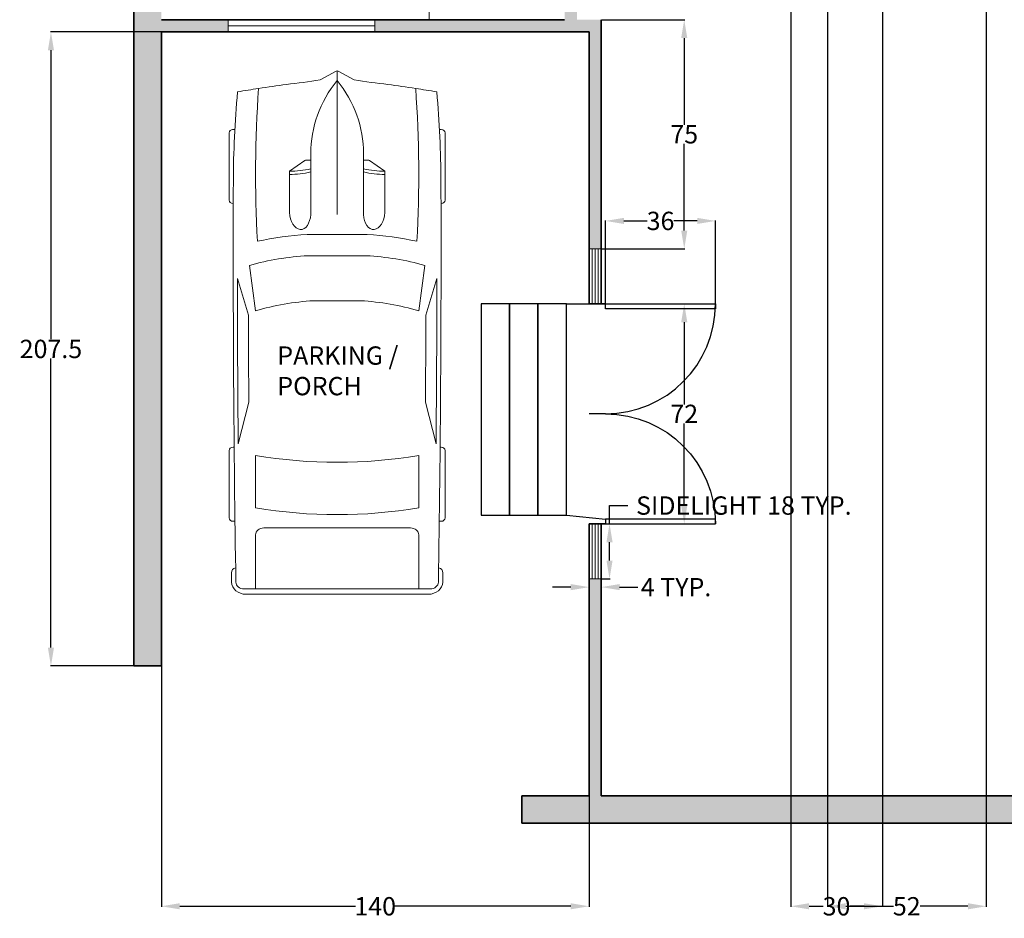
# Model space of a CAD drawing. Units: inches. Extents: x -16 to 578, y -553 to 49.
# Tile 1 of 5: x -14 to 308, y -553 to -259. Entities that reach past the tile are written whole.
import ezdxf

# ---------------------------------------------------------------- set-up
doc = ezdxf.new("R2010")
doc.units = ezdxf.units.IN
doc.header["$MEASUREMENT"] = 0
for name, color, linetype, lineweight in [('A-ANNO-DIMS', 2, 'Continuous', 18), ('A-AREA-IDEN', 7, 'Continuous', 25), ('A-DOOR', 3, 'Continuous', 25), ('A-FLOR-CASE', 8, 'Continuous', 18), ('A-FLOR-STRS', 7, 'Continuous', 25), ('A-GLAZ', 4, 'Continuous', 18), ('A-SITE-VEHC', 8, 'Continuous', 13), ('A-WALL', 7, 'Continuous', 35)]:
    doc.layers.add(name, color=color, linetype=linetype, lineweight=lineweight)
doc.layers.add('A-WALL-PATT', color=251, linetype='Continuous', lineweight=13, true_color=0x636466)
doc.styles.get("Standard").update_dxf_attribs({"font": 'arial.ttf'})
doc.dimstyles.get("Standard").update_dxf_attribs({"dimtxt": 6, "dimasz": 6, "dimexe": 0.18, "dimexo": 0.0625, "dimgap": 0.09, "dimtad": 0, "dimtih": 1, "dimtoh": 1, "dimdec": 0, "dimzin": 0, "dimdsep": 46, "dimlunit": 4, "dimtxsty": 'Standard', "dimcen": 0.09, "dimadec": 0, "dimazin": 0, "dimtfac": 1, "dimtdec": 0, "dimtofl": 0, "dimtmove": 0, "dimatfit": 3, "dimfxl": 1, "dimtolj": 1, "dimtzin": 0, "dimarcsym": 0})

# ---------------------------------------------------------------- blocks, each defined once
blk = doc.blocks.new('*U19')
for p, q in [((0, 0), (0, -6)), ((40, 0), (40, -6))]:
    blk.add_line(p, q)
blk.add_lwpolyline([(0, 0), (0, 40), (1.75, 40), (1.75, 0)], close=True)
blk.add_arc((0, 0), 40, 0, 90)
blk = doc.blocks.new('*U18')
for p, q in [((21.1, 37.41), (21.1, 36.83)), ((46.55, 38.89), (22.35, 38.89)), ((47.8, 37.39), (47.8, 37.41)), ((87.99, 31.87), (74.76, 35.92)), ((134.31, 35.6), (119.29, 31.78)), ((135.45, 37.07), (135.45, 37.41)), ((136.7, 38.89), (160.9, 38.89)), ((162.15, 37.41), (162.15, 36.77)), ((186.47, -33.5), (186.47, 33.5)), ((188.4, -32.76), (188.4, 32.76)), ((70.03, 31.54), (86.41, 29.35)), ((138.42, 29.35), (157.25, 29.35)), ((186.47, 29.35), (167.01, 29.35)), ((164.52, 26.39), (164.52, -26.39)), ((32.27, 11.63), (36.13, 17.17)), ((36.13, 17.17), (50.94, 17.17)), ((32.12, 9.51), (32.12, 11.15)), ((58.92, -10.77), (58.92, 10.77)), ((29.77, 9.51), (51.68, 9.51)), ((66.55, -10.53), (66.55, 10.53)), ((82.74, 8.5), (82.74, -8.5)), ((186.47, -10.53), (186.47, 10.53)), ((3.27, 6.13), (0.1, 0.41)), ((0, 0), (51.68, 0)), ((0.1, -0.41), (3.27, -6.13)), ((29.77, -9.51), (51.68, -9.51)), ((32.12, -9.51), (32.12, -11.15)), ((32.27, -11.63), (36.13, -17.17)), ((36.13, -17.17), (50.94, -17.17)), ((86.41, -29.35), (70.03, -31.54)), ((87.99, -31.87), (74.76, -35.92)), ((134.31, -35.6), (119.29, -31.78)), ((157.25, -29.35), (138.42, -29.35)), ((167.01, -29.35), (186.47, -29.35)), ((21.1, -37.41), (21.1, -36.83)), ((46.55, -38.89), (22.35, -38.89)), ((47.8, -37.39), (47.8, -37.41)), ((135.45, -37.07), (135.45, -37.41)), ((136.7, -38.89), (160.9, -38.89)), ((162.15, -37.41), (162.15, -36.77))]:
    blk.add_line(p, q)
for centre, major_axis, ratio, start_param, end_param in [((266.03, -27.52), (0, 313.31), 0.842304, 1.367076, 1.39176), ((41.19, -490.86), (0, 528.23), 0.842304, 0.00281, 0.075598), ((22.35, 37.41), (0, -1.48), 0.842304, 3.141593, 4.712389), ((64.48, -10555.62), (0, 10593.03), 0.842304, -0.013397, 0.002797), ((46.55, 37.41), (0, 1.48), 0.842304, -1.570796, 0), ((64.48, -10555.62), (0, -10591.55), 0.842304, 3.133765, 3.140441), ((136.7, 37.41), (0, -1.48), 0.842304, 3.141593, 4.712389), ((160.9, 37.41), (0, 1.48), 0.842304, -1.570796, 0), ((180.63, 35.84), (0, 2.22), 0.842304, -0.013017, 1.249894), ((64.48, -10556.36), (0, 10595.31), 0.842304, -0.013397, -0.013017), ((183.98, 33.5), (0, -2.96), 0.842304, 1.570796, 3.128196), ((183.98, 32.76), (0, -5.25), 0.842304, 1.570796, 3.128196), ((95.79, -3666.35), (0, -3698.24), 0.842304, 3.134049, 3.144098), ((37.47, -593.96), (0, -623.33), 0.842304, 3.096046, 3.200911), ((134.4, 5.39), (0, -89.78), 0.842304, 4.449482, 4.652344), ((135.29, 5.39), (0, 81.77), 0.842304, 1.245306, 1.50788), ((149.6, 2.8), (0, -79.58), 0.842304, 4.372215, 4.640744), ((17.08, 0), (0, 147.02), 0.842304, 4.511394, 4.913384), ((35.91, 0), (0, 147.02), 0.842304, 4.511394, 4.913384), ((167.01, 26.39), (0, 2.96), 0.842304, 0, 1.570796), ((259.18, -27.52), (0, -305.3), 0.842304, 4.528606, 4.561838), ((-204.49, 52.4), (0, -250.96), 0.842304, 1.385369, 1.434372), ((13.04, 17.01), (0, 27.42), 0.842304, 4.435146, 4.718221), ((14.2, 17.01), (0, 27.42), 0.842304, 4.435146, 4.718221), ((50.79, 13.34), (6.34, -0.36), 0.603834, -1.395552, 1.581315), ((32.75, 11.15), (0, 0.74), 0.842304, 0.879714, 1.570796), ((29.77, -46.66), (0, 56.17), 0.842304, 0, 0.590319), ((0.62, 0), (0, -0.74), 0.842304, 4.131459, 5.293319), ((29.77, 46.66), (0, 56.17), 0.842304, 2.551274, 3.141593), ((-204.49, -52.4), (0, 250.96), 0.842304, -1.434372, -1.385369), ((13.04, -17.01), (0, -27.42), 0.842304, 1.564964, 1.848039), ((14.2, -17.01), (0, -27.42), 0.842304, 1.564964, 1.848039), ((135.29, -5.39), (0, -81.77), 0.842304, -1.50788, -1.245306), ((149.6, -2.8), (0, -79.58), 0.842304, -1.499151, -1.230623), ((32.75, -11.15), (0, -0.74), 0.842304, 4.712389, 5.403472), ((134.4, -5.39), (0, -89.78), 0.842304, -1.510751, -1.307889), ((259.18, 27.52), (0, 305.3), 0.842304, 1.721348, 1.754579), ((266.03, 27.52), (0, 313.31), 0.842304, 1.749832, 1.774517), ((37.47, 593.96), (0, -623.33), 0.842304, -0.059319, 0.045547), ((167.01, -26.39), (0, -2.96), 0.842304, 4.712389, 6.283185), ((95.79, 3666.35), (0, -3698.24), 0.842304, -0.002505, 0.007544), ((183.98, -33.5), (0, 2.96), 0.842304, 3.15499, 4.712389), ((183.98, -32.76), (0, -5.25), 0.842304, 0.013397, 1.570796), ((41.19, 490.86), (0, -528.23), 0.842304, -0.075598, -0.00281), ((22.35, -37.41), (0, 1.48), 0.842304, 1.570796, 3.141593), ((64.48, 10555.62), (0, 10593.03), 0.842304, 3.138796, 3.15499), ((46.55, -37.41), (0, -1.48), 0.842304, 0, 1.570796), ((64.48, 10555.62), (0, -10591.55), 0.842304, 0.001152, 0.007828), ((136.7, -37.41), (0, -1.48), 0.842304, -1.570796, 0), ((160.9, -37.41), (0, 1.48), 0.842304, 3.141593, 4.712389), ((180.63, -35.84), (0, -2.22), 0.842304, -1.249894, 0.013017), ((64.48, 10556.36), (0, 10595.31), 0.842304, 3.15461, 3.15499)]:
    blk.add_ellipse(centre, major_axis=major_axis, ratio=ratio, start_param=start_param, end_param=end_param)
at = {"extrusion": (0, 0, -1)}
blk.add_ellipse((50.79, -13.34), major_axis=(6.34, 0.36), ratio=0.603834, start_param=-1.395552, end_param=1.581315, dxfattribs=at)
blk = doc.blocks.new('SIDELIGHT-18X4')
for p, q in [((1, 18), (1, 0)), ((2, 18), (2, 0)), ((3, 18), (3, 0))]:
    blk.add_line(p, q)
blk.add_lwpolyline([(0, 0), (0, 18), (4, 18), (4, 0)], close=True)
blk = doc.blocks.new('*D50')
at = {"layer": 'A-ANNO-DIMS', "color": 0, "lineweight": -2, "transparency": 16777216}
for p, q in [((178.89, -423.77), (178.89, -417.77)), ((178.89, -417.77), (184.89, -417.77)), ((176.25, -423.77), (179.07, -423.77)), ((178.89, -435.77), (178.89, -429.77)), ((176.25, -441.77), (179.07, -441.77))]:
    blk.add_line(p, q, dxfattribs=at)
at = {"layer": 'A-ANNO-DIMS', "color": 0, "transparency": 16777216}
for points in [[(177.89, -429.77), (179.89, -429.77), (178.89, -423.77)], [(177.89, -435.77), (179.89, -435.77), (178.89, -441.77)]]:
    blk.add_solid(points, dxfattribs=at)
at = {"layer": 'Defpoints', "color": 0, "transparency": 16777216}
for p in [(176.19, -423.77), (178.89, -423.77), (176.19, -441.77)]:
    blk.add_point(p, dxfattribs=at)
at = {"layer": 'A-ANNO-DIMS', "color": 0, "transparency": 16777216, "insert": (222.85, -417.77), "char_height": 6, "attachment_point": 5}
blk.add_mtext('\\A1;SIDELIGHT 18 TYP.', dxfattribs=at)
blk = doc.blocks.new('*D51')
at = {"layer": 'A-ANNO-DIMS', "color": 0, "lineweight": -2, "transparency": 16777216}
for p, q in [((166.19, -444.47), (160.19, -444.47)), ((172.19, -441.83), (172.19, -444.65)), ((176.19, -441.83), (176.19, -444.65)), ((182.19, -444.47), (188.19, -444.47))]:
    blk.add_line(p, q, dxfattribs=at)
at = {"layer": 'A-ANNO-DIMS', "color": 0, "transparency": 16777216}
for points in [[(166.19, -443.47), (166.19, -445.47), (172.19, -444.47)], [(182.19, -443.47), (182.19, -445.47), (176.19, -444.47)]]:
    blk.add_solid(points, dxfattribs=at)
at = {"layer": 'Defpoints', "color": 0, "transparency": 16777216}
for p in [(172.19, -441.77), (176.19, -441.77), (176.19, -444.47)]:
    blk.add_point(p, dxfattribs=at)
at = {"layer": 'A-ANNO-DIMS', "color": 0, "transparency": 16777216, "insert": (200.67, -444.47), "char_height": 6, "attachment_point": 5}
blk.add_mtext('\\A1;4 TYP.', dxfattribs=at)
blk = doc.blocks.new('*D64')
at = {"layer": 'A-ANNO-DIMS', "color": 0, "lineweight": -2, "transparency": 16777216}
for p, q in [((172.19, -441.83), (172.19, -549.1)), ((32.19, -470.34), (32.19, -549.1)), ((38.19, -548.92), (95.76, -548.92)), ((166.19, -548.92), (108.61, -548.92))]:
    blk.add_line(p, q, dxfattribs=at)
at = {"layer": 'A-ANNO-DIMS', "color": 0, "transparency": 16777216}
for points in [[(38.19, -547.92), (38.19, -549.92), (32.19, -548.92)], [(166.19, -547.92), (166.19, -549.92), (172.19, -548.92)]]:
    blk.add_solid(points, dxfattribs=at)
at = {"layer": 'Defpoints', "color": 0, "transparency": 16777216}
for p in [(172.19, -441.77), (32.19, -470.28), (172.19, -548.92)]:
    blk.add_point(p, dxfattribs=at)
at = {"layer": 'A-ANNO-DIMS', "color": 0, "transparency": 16777216, "insert": (102.19, -548.92), "char_height": 6, "attachment_point": 5}
blk.add_mtext('\\A1;140', dxfattribs=at)
blk = doc.blocks.new('*D65')
at = {"layer": 'A-ANNO-DIMS', "color": 0, "lineweight": -2, "transparency": 16777216}
for p, q in [((32.13, -262.77), (-4.14, -262.77)), ((-3.96, -268.77), (-3.96, -363.37)), ((-3.96, -464.28), (-3.96, -369.68)), ((32.13, -470.28), (-4.14, -470.28))]:
    blk.add_line(p, q, dxfattribs=at)
at = {"layer": 'A-ANNO-DIMS', "color": 0, "transparency": 16777216}
for points in [[(-4.96, -268.77), (-2.96, -268.77), (-3.96, -262.77)], [(-4.96, -464.28), (-2.96, -464.28), (-3.96, -470.28)]]:
    blk.add_solid(points, dxfattribs=at)
at = {"layer": 'Defpoints', "color": 0, "transparency": 16777216}
for p in [(32.19, -262.77), (-3.96, -470.28), (32.19, -470.28)]:
    blk.add_point(p, dxfattribs=at)
at = {"layer": 'A-ANNO-DIMS', "color": 0, "transparency": 16777216, "insert": (-3.96, -366.52), "char_height": 6, "attachment_point": 5}
blk.add_mtext('\\A1;207.5', dxfattribs=at)
blk = doc.blocks.new('*D66')
at = {"layer": 'A-ANNO-DIMS', "color": 0, "lineweight": -2, "transparency": 16777216}
for p, q in [((176.25, -351.77), (203.52, -351.77)), ((203.34, -357.77), (203.34, -384.66)), ((203.34, -417.77), (203.34, -390.87)), ((176.25, -423.77), (203.52, -423.77))]:
    blk.add_line(p, q, dxfattribs=at)
at = {"layer": 'A-ANNO-DIMS', "color": 0, "transparency": 16777216}
for points in [[(202.34, -357.77), (204.34, -357.77), (203.34, -351.77)], [(202.34, -417.77), (204.34, -417.77), (203.34, -423.77)]]:
    blk.add_solid(points, dxfattribs=at)
at = {"layer": 'Defpoints', "color": 0, "transparency": 16777216}
for p in [(176.19, -351.77), (176.19, -423.77), (203.34, -423.77)]:
    blk.add_point(p, dxfattribs=at)
at = {"layer": 'A-ANNO-DIMS', "color": 0, "transparency": 16777216, "insert": (203.34, -387.77), "char_height": 6, "attachment_point": 5}
blk.add_mtext('\\A1;72', dxfattribs=at)
blk = doc.blocks.new('*D67')
at = {"layer": 'A-ANNO-DIMS', "color": 0, "lineweight": -2, "transparency": 16777216}
for p, q in [((177.59, -351.7), (177.59, -324.44)), ((183.59, -324.62), (191.2, -324.62)), ((207.59, -324.62), (199.97, -324.62)), ((213.59, -351.7), (213.59, -324.44))]:
    blk.add_line(p, q, dxfattribs=at)
at = {"layer": 'A-ANNO-DIMS', "color": 0, "transparency": 16777216}
for points in [[(183.59, -323.62), (183.59, -325.62), (177.59, -324.62)], [(207.59, -323.62), (207.59, -325.62), (213.59, -324.62)]]:
    blk.add_solid(points, dxfattribs=at)
at = {"layer": 'Defpoints', "color": 0, "transparency": 16777216}
for p in [(213.59, -324.62), (177.59, -351.77), (213.59, -351.77)]:
    blk.add_point(p, dxfattribs=at)
at = {"layer": 'A-ANNO-DIMS', "color": 0, "transparency": 16777216, "insert": (195.59, -324.62), "char_height": 6, "attachment_point": 5}
blk.add_mtext('\\A1;36', dxfattribs=at)
blk = doc.blocks.new('*D68')
at = {"layer": 'A-ANNO-DIMS', "color": 0, "lineweight": -2, "transparency": 16777216}
for p, q in [((176.25, -258.77), (203.52, -258.77)), ((203.34, -264.77), (203.34, -293.13)), ((203.34, -327.77), (203.34, -299.41)), ((176.25, -333.77), (203.52, -333.77))]:
    blk.add_line(p, q, dxfattribs=at)
at = {"layer": 'A-ANNO-DIMS', "color": 0, "transparency": 16777216}
for points in [[(202.34, -264.77), (204.34, -264.77), (203.34, -258.77)], [(202.34, -327.77), (204.34, -327.77), (203.34, -333.77)]]:
    blk.add_solid(points, dxfattribs=at)
at = {"layer": 'Defpoints', "color": 0, "transparency": 16777216}
for p in [(176.19, -258.77), (176.19, -333.77), (203.34, -333.77)]:
    blk.add_point(p, dxfattribs=at)
at = {"layer": 'A-ANNO-DIMS', "color": 0, "transparency": 16777216, "insert": (203.34, -296.27), "char_height": 6, "attachment_point": 5}
blk.add_mtext('\\A1;75', dxfattribs=at)
blk = doc.blocks.new('*D81')
at = {"layer": 'A-ANNO-DIMS', "color": 0, "lineweight": -2, "transparency": 16777216}
for p, q in [((238.19, -72.83), (238.19, -549.1)), ((268.19, -72.83), (268.19, -549.1)), ((244.19, -548.92), (248.81, -548.92)), ((262.19, -548.92), (257.56, -548.92))]:
    blk.add_line(p, q, dxfattribs=at)
at = {"layer": 'A-ANNO-DIMS', "color": 0, "transparency": 16777216}
for points in [[(244.19, -547.92), (244.19, -549.92), (238.19, -548.92)], [(262.19, -547.92), (262.19, -549.92), (268.19, -548.92)]]:
    blk.add_solid(points, dxfattribs=at)
at = {"layer": 'Defpoints', "color": 0, "transparency": 16777216}
for p in [(238.19, -72.77), (268.19, -72.77), (268.19, -548.92)]:
    blk.add_point(p, dxfattribs=at)
at = {"layer": 'A-ANNO-DIMS', "color": 0, "transparency": 16777216, "insert": (253.19, -548.92), "char_height": 6, "attachment_point": 5}
blk.add_mtext('\\A1;30', dxfattribs=at)
blk = doc.blocks.new('*D82')
at = {"layer": 'A-ANNO-DIMS', "color": 0, "lineweight": -2, "transparency": 16777216}
for p, q in [((250.19, -102.83), (250.19, -549.1)), ((302.19, -102.91), (302.19, -549.1)), ((256.19, -548.92), (271.83, -548.92)), ((296.19, -548.92), (280.54, -548.92))]:
    blk.add_line(p, q, dxfattribs=at)
at = {"layer": 'A-ANNO-DIMS', "color": 0, "transparency": 16777216}
for points in [[(256.19, -547.92), (256.19, -549.92), (250.19, -548.92)], [(296.19, -547.92), (296.19, -549.92), (302.19, -548.92)]]:
    blk.add_solid(points, dxfattribs=at)
at = {"layer": 'Defpoints', "color": 0, "transparency": 16777216}
for p in [(250.19, -102.77), (302.19, -102.85), (302.19, -548.92)]:
    blk.add_point(p, dxfattribs=at)
at = {"layer": 'A-ANNO-DIMS', "color": 0, "transparency": 16777216, "insert": (276.19, -548.92), "char_height": 6, "attachment_point": 5}
blk.add_mtext('\\A1;52', dxfattribs=at)

msp = doc.modelspace()

# ---------------------------------------------------------------- hatches: boundary and pattern name
at = {"layer": 'A-WALL-PATT'}
h = msp.add_hatch(color=256, dxfattribs=at)
h.dxf.hatch_style = 1
h.paths.add_polyline_path([(32.1882, 9.2337), (89.8211, 9.2337), (89.8211, 18.2337), (23.1882, 18.2337), (23.1882, -55.5259), (32.1882, -55.5259)])
h.paths.add_polyline_path([(219.6411, 18.2337), (137.8211, 18.2337), (137.8211, 9.2337), (146.4179, 9.2337), (188.1882, 9.2337), (188.1882, -98.7663), (192.1882, -98.7663), (192.1882, -72.7663), (238.1882, -72.7663), (238.1882, -68.7663), (192.1882, -68.7663), (192.1882, 9.2337), (219.6411, 9.2337)])
h.paths.add_polyline_path([(307.3924, 18.2337), (243.6411, 18.2337), (243.6411, 9.2337), (274.1882, 9.2337), (274.1882, -26.7663), (274.1882, -68.7663), (268.1882, -68.7663), (268.1882, -72.7663), (274.1882, -72.7663), (274.1882, -98.7663), (250.1882, -98.7663), (250.1882, -102.7663), (274.1882, -102.7663), (278.1882, -102.7663), (302.188, -102.8481), (302.188, -98.8481), (278.1882, -98.7663), (278.1882, -86.8559, -0.01827889), (278.1882, -85.7663), (278.1882, -72.7663), (284.1882, -72.7663), (284.1882, -68.7663), (278.1882, -68.7663), (278.1882, 9.2337), (307.3924, 9.2337)])
h.paths.add_polyline_path([(402.6701, 18.2337), (331.3924, 18.2337), (331.3924, 9.2337), (358.1882, 9.2337), (358.1882, -26.7663), (358.1882, -68.7663), (314.1882, -68.7663), (314.1882, -72.7663), (358.1882, -72.7663), (358.1882, -98.7663), (362.1882, -98.7663), (362.1882, 9.2337), (402.6701, 9.2337)])
h.paths.add_polyline_path([(503.1882, 18.2337), (450.6701, 18.2337), (450.6701, 9.2337), (462.8072, 9.2337), (494.1882, 9.2337), (494.1882, -38.053), (503.1882, -38.053)])
h.paths.add_polyline_path([(503.1882, -86.053), (494.1882, -86.053), (494.1882, -134.7663), (362.1882, -134.7663), (362.1882, -128.7663), (358.1882, -128.7663), (358.1882, -138.7663), (358.1882, -234.7663), (362.1882, -234.7663), (362.1882, -138.7663), (494.1882, -138.7663), (494.1882, -181.1501), (503.1882, -181.1501)])
h.paths.add_polyline_path([(503.1882, -229.1501), (494.1882, -229.1501), (494.1882, -270.7663), (362.1882, -270.7663), (362.1882, -264.7663), (358.1882, -264.7663), (358.1882, -294.7663), (358.1882, -323.1753), (362.1882, -323.1753), (362.1882, -298.7663), (362.1882, -294.7663), (362.1882, -274.7663), (494.1882, -274.7663), (494.1882, -294.7663), (494.1882, -298.7663), (494.1882, -310.411), (503.1882, -310.411)])
h.paths.add_polyline_path([(503.1882, -358.411), (494.1882, -358.411), (494.1882, -394.7663), (362.1882, -394.7663), (362.1882, -353.1753), (358.1882, -353.1753), (358.1882, -398.7663), (494.1882, -398.7663), (494.1882, -512.7663), (451.8049, -512.7663), (451.8049, -521.7663), (503.1882, -521.7663)])
h.paths.add_polyline_path([(403.8049, -512.7663), (176.1882, -512.7663), (176.1882, -441.7663), (172.1882, -441.7663), (172.1882, -512.7663), (150.1882, -512.7663), (150.1882, -521.7663), (403.8049, -521.7663)])
h.paths.add_polyline_path([(176.1882, -258.7663), (168.1882, -258.7663), (168.1882, -246.7663), (168.1882, -234.7663), (168.1882, -222.7663), (164.1882, -222.7663), (164.1882, -234.7663), (164.1882, -258.7663), (102.0641, -258.7663), (102.0641, -262.7663), (168.1882, -262.7663), (172.1882, -262.7663), (172.1882, -333.7663), (176.1882, -333.7663), (176.1882, -262.7663)])
h.paths.add_polyline_path([(32.1882, -262.7663), (54.0641, -262.7663), (54.0641, -258.7663), (32.1882, -258.7663), (32.1882, -229.1501), (23.1882, -229.1501), (23.1882, -283.4909), (23.1882, -470.2771), (32.1882, -470.2771), (32.1882, -283.4909)])
h.paths.add_polyline_path([(32.1882, -103.5259), (23.1882, -103.5259), (23.1882, -181.1501), (32.1882, -181.1501)])
h.paths.add_polyline_path([(192.1882, -128.7663), (188.1882, -128.7663), (188.1882, -134.7663), (32.1882, -134.7663), (32.1882, -138.7663), (164.1882, -138.7663), (164.1882, -162.7663), (164.1882, -174.7663), (168.1882, -174.7663), (168.1882, -162.7663), (168.1882, -138.7663), (192.1882, -138.7663)])

# ---------------------------------------------------------------- linework, layer by layer
at = {"layer": 'A-FLOR-CASE'}
msp.add_line((119.8061, -234.7663), (119.8061, -258.7663), dxfattribs=at)
at = {"layer": 'A-FLOR-STRS'}
for p, q in [((164.7625, -351.7663), (172.1882, -351.7663)), ((164.7625, -420.9713), (177.5882, -422.1913))]:
    msp.add_line(p, q, dxfattribs=at)
for points in [[(146.1767, -351.7663), (136.8838, -351.7663), (136.8838, -420.9713), (146.1767, -420.9713)], [(155.4696, -351.7663), (146.1767, -351.7663), (146.1767, -420.9713), (155.4696, -420.9713)], [(164.7625, -351.7663), (155.4696, -351.7663), (155.4696, -420.9713), (164.7625, -420.9713)]]:
    msp.add_lwpolyline(points, close=True, dxfattribs=at)
at = {"layer": 'A-GLAZ'}
msp.add_line((54.0641, -262.7663), (102.0641, -262.7663), dxfattribs=at)
for points in [[(102.0641, -258.7663), (102.0641, -262.7663), (54.0641, -262.7663), (54.0641, -258.7663)], [(54.0641, -260.7663), (102.0641, -260.7663)]]:
    msp.add_lwpolyline(points, close=True, dxfattribs=at)
at = {"layer": 'A-WALL'}
for p, q in [((32.1882, -258.7663), (164.1882, -258.7663)), ((176.1882, -258.7663), (176.1882, -262.7663)), ((32.1882, -283.4909), (32.1882, -262.7663)), ((32.1882, -262.7663), (124.1882, -262.7663)), ((102.0641, -262.7663), (168.1882, -262.7663)), ((168.1882, -262.7663), (172.1882, -262.7663)), ((172.1882, -351.7663), (172.1882, -262.7663)), ((176.1882, -351.7663), (176.1882, -262.7663)), ((23.1882, -470.2771), (23.1882, -283.4909)), ((32.1882, -283.4909), (32.1882, -470.2771)), ((176.1882, -351.7663), (172.1882, -351.7663)), ((172.1882, -512.7663), (172.1882, -423.7663)), ((176.1882, -423.7663), (172.1882, -423.7663)), ((176.1882, -512.7663), (176.1882, -423.7663)), ((32.1882, -470.2771), (23.1882, -470.2771)), ((172.1882, -512.7663), (150.1882, -512.7663)), ((172.1882, -512.7663), (150.1882, -512.7663)), ((150.1882, -512.7663), (150.1882, -521.7663)), ((494.1882, -512.7663), (176.1882, -512.7663)), ((358.1882, -512.7663), (176.1882, -512.7663))]:
    msp.add_line(p, q, dxfattribs=at)
msp.add_lwpolyline([(23.1882, -283.4909), (23.1882, 18.2337), (503.1882, 18.2337), (503.1882, -521.7663), (150.1882, -521.7663)], dxfattribs=at)

# ---------------------------------------------------------------- block references
at = {"layer": 'A-DOOR', "yscale": 0.9, "zscale": 0.9, "rotation": 270}
for p, xscale in [((177.5882, -351.7663), 0.9), ((177.5882, -423.7663), -0.9)]:
    msp.add_blockref('*U19', p, dxfattribs=dict(at, xscale=xscale))
at = {"layer": 'A-GLAZ'}
for p in [(172.1882, -351.7663), (172.1882, -441.7663)]:
    msp.add_blockref('SIDELIGHT-18X4', p, dxfattribs=at)
at = {"layer": 'A-SITE-VEHC', "xscale": 0.9093012667829208, "yscale": 0.9093012667829208, "zscale": 0.9093012667829208, "rotation": 270}
msp.add_blockref('*U18', (89.7284, -275.4912), dxfattribs=at)

# ---------------------------------------------------------------- texts
at = {"layer": 'A-AREA-IDEN', "insert": (70.131, -365.6842), "char_height": 6, "attachment_point": 1}
msp.add_mtext_dynamic_manual_height_columns('PARKING /\\PPORCH', width=73.245661, gutter_width=1, heights=[0], dxfattribs=at)

# ---------------------------------------------------------------- dimensions: what is measured, and where the dimension line sits
at = {"layer": 'A-ANNO-DIMS'}
for base, p1, p2, picture, middle in [((268.1882, -548.9163), (238.1882, -72.7663), (268.1882, -72.7663), '*D81', (253.1882, -548.9163)), ((302.188, -548.9163), (250.1882, -102.7663), (302.188, -102.8481), '*D82', (276.1881, -548.9163)), ((213.5882, -324.6163), (177.5882, -351.7663), (213.5882, -351.7663), '*D67', (195.5882, -324.6163)), ((172.1882, -548.9163), (32.1882, -470.2771), (172.1882, -441.7663), '*D64', (102.1882, -548.9163))]:
    dim = msp.add_linear_dim(base=base, p1=p1, p2=p2, dimstyle='Standard', override={"dimdec": 0, "dimlfac": 1, "dimrnd": 0, "dimzin": 0, "dimdsep": 46, "dimlunit": 2}, dxfattribs=at)
    dim.commit()
    dim.dimension.update_dxf_attribs({"geometry": picture, "text_midpoint": middle})
for base, p1, p2, angle, override, picture, middle in [((203.3382, -333.7663), (176.1882, -258.7663), (176.1882, -333.7663), 270, {"dimdec": 0, "dimlfac": 1, "dimrnd": 0, "dimzin": 0, "dimdsep": 46, "dimlunit": 2}, '*D68', (203.3382, -296.2663)), ((-3.9618, -470.2771), (32.1882, -262.7663), (32.1882, -470.2771), 90, {"dimdec": 1, "dimlfac": 1, "dimrnd": 0, "dimzin": 0, "dimdsep": 46, "dimlunit": 2}, '*D65', (-3.9618, -366.5217)), ((203.3382, -423.7663), (176.1882, -351.7663), (176.1882, -423.7663), 270, {"dimdec": 0, "dimlfac": 1, "dimrnd": 0, "dimzin": 0, "dimdsep": 46, "dimlunit": 2}, '*D66', (203.3382, -387.7663))]:
    dim = msp.add_linear_dim(base=base, p1=p1, p2=p2, angle=angle, dimstyle='Standard', override=override, dxfattribs=at)
    dim.commit()
    dim.dimension.update_dxf_attribs({"geometry": picture, "text_midpoint": middle})
dim = msp.add_linear_dim(base=(178.8882, -423.7663), p1=(176.1882, -441.7663), p2=(176.1882, -423.7663), angle=90, text='SIDELIGHT <> TYP.', dimstyle='Standard', override={"dimdec": 0, "dimlfac": 1, "dimrnd": 0, "dimzin": 0, "dimdsep": 46, "dimlunit": 2}, dxfattribs=at)
dim.commit()
dim.dimension.update_dxf_attribs({"geometry": '*D50', "text_midpoint": (222.8547, -417.7663)})
dim = msp.add_linear_dim(base=(176.1882, -444.4663), p1=(172.1882, -441.7663), p2=(176.1882, -441.7663), text='<> TYP.', dimstyle='Standard', override={"dimdec": 0, "dimlfac": 1, "dimrnd": 0, "dimzin": 0, "dimdsep": 46, "dimlunit": 2}, dxfattribs=at)
dim.commit()
dim.dimension.update_dxf_attribs({"geometry": '*D51', "text_midpoint": (200.6711, -444.4663)})

doc.saveas('drawing.dxf')
